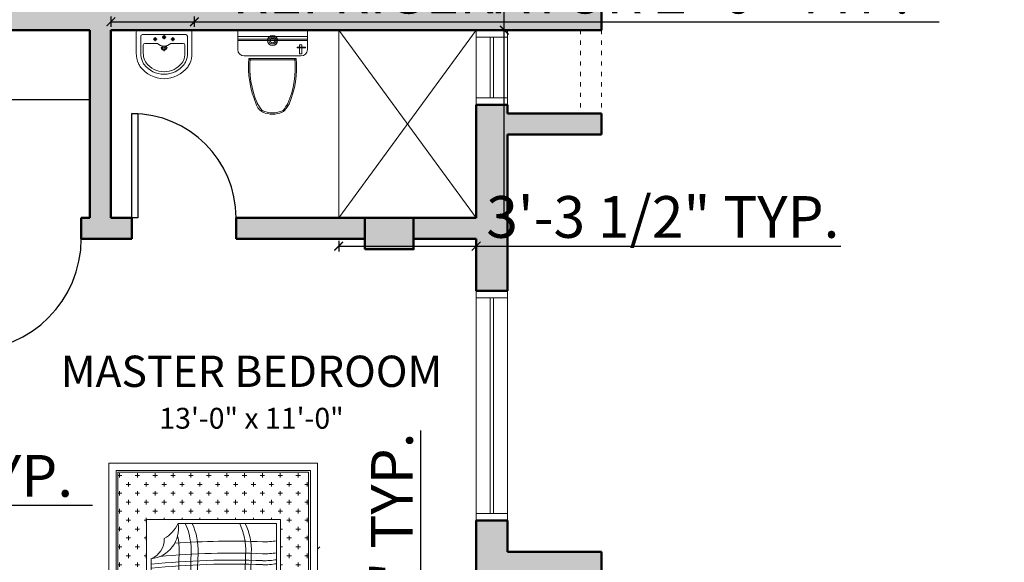
# Model space of a CAD drawing. Units: inches. Extents: x 375 to 1122, y 27 to 1069.
# Tile 151 of 155: x 819 to 1102, y 716 to 872. Entities that reach past the tile are written whole.
import ezdxf

# ---------------------------------------------------------------- set-up
doc = ezdxf.new("R2010")
doc.units = ezdxf.units.IN
doc.linetypes.add('ACAD_ISO03W100', pattern=[30, 12, -18])
for name, color, linetype, lineweight in [('A-ANNO-DIMS', 2, 'Continuous', 18), ('A-AREA-IDEN', 7, 'Continuous', 18), ('A-COLS-PATT', 10, 'Continuous', 13), ('A-FLOR-FIXT', 55, 'Continuous', 18), ('A-FLOR-MILL', 55, 'Continuous', 25), ('A-WALL-OVHD', 77, 'ACAD_ISO03W100', 18), ('A-WALL-PATT', 252, 'Continuous', 13), ('Columns', 10, 'Continuous', 50), ('Doors', 150, 'Continuous', 25), ('Furniture', 30, 'Continuous', 18), ('Shower Areas', 53, 'Continuous', 18), ('Walls', 250, 'Continuous', 50), ('Windows', 122, 'Continuous', 18)]:
    doc.layers.add(name, color=color, linetype=linetype, lineweight=lineweight)
doc.styles.get("Standard").update_dxf_attribs({"font": 'arial.ttf'})
doc.dimstyles.new('ISO-25', dxfattribs={"dimtxt": 12, "dimasz": 2.5, "dimexe": 1.5, "dimexo": 1.5, "dimtad": 1, "dimdec": 1, "dimlunit": 3, "dimtxsty": 'Standard', "dimblk": 'ARCHTICK', "dimcen": 2.5, "dimadec": 0, "dimazin": 0, "dimtfac": 1, "dimtdec": 1, "dimtmove": 0, "dimatfit": 3, "dimfxl": 1.5, "dimfxlon": 1, "dimarcsym": 0})

# ---------------------------------------------------------------- blocks, each defined once
blk = doc.blocks.new('*U2')
for p, q in [((0, 0), (0, 4)), ((32, 0), (32, 4))]:
    blk.add_line(p, q)
blk.add_lwpolyline([(0, 0), (0, -32), (1.75, -32), (1.75, 0)], close=True)
blk.add_arc((0, 0), 32, 270, 0)
blk = doc.blocks.new('*U3')
for p, q in [((0, 0), (0, -4)), ((30, 0), (30, -4))]:
    blk.add_line(p, q)
blk.add_lwpolyline([(0, 0), (0, 30), (1.75, 30), (1.75, 0)], close=True)
blk.add_arc((0, 0), 30, 0, 90)
blk = doc.blocks.new('A$C52B64FF5')
for p, q in [((0.522, 2.628), (0, 2.628)), ((0, 2.628), (0, 2.178)), ((0.262, 2.403), (0.262, 2.616)), ((0.522, 2.178), (0.522, 2.628)), ((2.022, 2.628), (0.522, 2.628)), ((0.522, 2.628), (0.522, 0.628)), ((2.543, 2.628), (2.022, 2.628)), ((2.022, 0.628), (2.022, 2.628)), ((2.022, 2.628), (2.022, 2.178)), ((2.282, 2.403), (2.282, 2.616)), ((2.543, 2.178), (2.543, 2.628)), ((0.721, 2.493), (0.692, 2.493)), ((0.692, 2.493), (0.692, 2.353)), ((0.721, 2.353), (0.721, 2.493)), ((1.767, 2.353), (1.767, 2.493)), ((1.767, 2.493), (1.796, 2.493)), ((1.796, 2.493), (1.796, 2.353)), ((0.263, 2.403), (0.023, 2.403)), ((0.023, 2.403), (0.5, 2.403)), ((0.263, 2.195), (0.263, 2.403)), ((0.692, 2.353), (0.721, 2.353)), ((1.796, 2.353), (1.767, 2.353)), ((2.52, 2.403), (2.043, 2.403)), ((2.28, 2.213), (2.28, 2.403)), ((2.28, 2.403), (2.52, 2.403)), ((0.575, 1.068), (0.575, 2.254)), ((0.575, 2.254), (1.978, 2.254)), ((1.978, 2.254), (1.978, 0.675)), ((0, 2.178), (0.522, 2.178)), ((0.093, 2.178), (0.101, 2.17)), ((0.101, 0), (0.101, 2.178)), ((0.181, 0.08), (0.181, 2.178)), ((0.201, 0.1), (0.201, 2.178)), ((0.201, 2.136), (0.245, 2.136)), ((0.22, 2.111), (0.22, 2.161)), ((0.395, 2.136), (0.445, 2.136)), ((0.42, 2.111), (0.42, 2.161)), ((2.543, 2.178), (2.022, 2.178)), ((2.022, 2.178), (2.543, 2.178)), ((2.022, 2.136), (2.045, 2.136)), ((2.195, 2.136), (2.245, 2.136)), ((2.22, 2.111), (2.22, 2.161)), ((2.337, 2.178), (2.337, 0.1)), ((2.357, 2.178), (2.357, 0.08)), ((2.437, 2.178), (2.437, 0)), ((0.295, 2.036), (0.345, 2.036)), ((0.32, 2.011), (0.32, 2.061)), ((0.495, 2.036), (0.522, 2.036)), ((0.52, 2.011), (0.52, 2.061)), ((2.095, 2.036), (2.145, 2.036)), ((2.12, 2.011), (2.12, 2.061)), ((2.295, 2.036), (2.337, 2.036)), ((2.32, 2.011), (2.32, 2.061)), ((0.201, 1.936), (0.245, 1.936)), ((0.22, 1.911), (0.22, 1.961)), ((0.395, 1.936), (0.445, 1.936)), ((0.42, 1.911), (0.42, 1.961)), ((2.022, 1.936), (2.045, 1.936)), ((2.195, 1.936), (2.245, 1.936)), ((2.22, 1.911), (2.22, 1.961)), ((0.295, 1.836), (0.345, 1.836)), ((0.32, 1.811), (0.32, 1.861)), ((0.495, 1.836), (0.522, 1.836)), ((0.52, 1.811), (0.52, 1.861)), ((2.095, 1.836), (2.145, 1.836)), ((2.12, 1.811), (2.12, 1.861)), ((2.295, 1.836), (2.337, 1.836)), ((2.32, 1.811), (2.32, 1.861)), ((0.201, 1.736), (0.245, 1.736)), ((0.22, 1.711), (0.22, 1.761)), ((0.32, 1.611), (0.32, 1.661)), ((0.395, 1.736), (0.445, 1.736)), ((0.42, 1.711), (0.42, 1.761)), ((0.52, 1.611), (0.52, 1.661)), ((2.022, 1.736), (2.045, 1.736)), ((2.12, 1.611), (2.12, 1.661)), ((2.195, 1.736), (2.245, 1.736)), ((2.22, 1.711), (2.22, 1.761)), ((2.32, 1.611), (2.32, 1.661)), ((0.22, 1.511), (0.22, 1.561)), ((0.295, 1.636), (0.345, 1.636)), ((0.42, 1.511), (0.42, 1.561)), ((0.495, 1.636), (0.522, 1.636)), ((2.095, 1.636), (2.145, 1.636)), ((2.22, 1.511), (2.22, 1.561)), ((2.295, 1.636), (2.337, 1.636)), ((0.201, 1.536), (0.245, 1.536)), ((0.295, 1.436), (0.345, 1.436)), ((0.32, 1.411), (0.32, 1.461)), ((0.395, 1.536), (0.445, 1.536)), ((0.495, 1.436), (0.522, 1.436)), ((0.52, 1.411), (0.52, 1.461)), ((2.022, 1.536), (2.045, 1.536)), ((2.095, 1.436), (2.145, 1.436)), ((2.12, 1.411), (2.12, 1.461)), ((2.195, 1.536), (2.245, 1.536)), ((2.295, 1.436), (2.337, 1.436)), ((2.32, 1.411), (2.32, 1.461)), ((0.201, 1.336), (0.245, 1.336)), ((0.22, 1.311), (0.22, 1.361)), ((0.395, 1.336), (0.445, 1.336)), ((0.42, 1.311), (0.42, 1.361)), ((2.022, 1.336), (2.045, 1.336)), ((2.195, 1.336), (2.245, 1.336)), ((2.22, 1.311), (2.22, 1.361)), ((0.295, 1.236), (0.345, 1.236)), ((0.32, 1.211), (0.32, 1.261)), ((0.495, 1.236), (0.522, 1.236)), ((0.52, 1.211), (0.52, 1.261)), ((2.095, 1.236), (2.145, 1.236)), ((2.12, 1.211), (2.12, 1.261)), ((2.295, 1.236), (2.337, 1.236)), ((2.32, 1.211), (2.32, 1.261)), ((0.201, 1.136), (0.245, 1.136)), ((0.22, 1.111), (0.22, 1.161)), ((0.395, 1.136), (0.445, 1.136)), ((0.42, 1.111), (0.42, 1.161)), ((2.022, 1.136), (2.045, 1.136)), ((2.195, 1.136), (2.245, 1.136)), ((2.22, 1.111), (2.22, 1.161)), ((0.295, 1.036), (0.345, 1.036)), ((0.32, 1.011), (0.32, 1.061)), ((0.495, 1.036), (0.522, 1.036)), ((0.52, 1.011), (0.52, 1.061)), ((2.095, 1.036), (2.145, 1.036)), ((2.12, 1.011), (2.12, 1.061)), ((2.295, 1.036), (2.337, 1.036)), ((2.32, 1.011), (2.32, 1.061)), ((0.201, 0.936), (0.245, 0.936)), ((0.22, 0.911), (0.22, 0.961)), ((0.395, 0.936), (0.445, 0.936)), ((0.42, 0.911), (0.42, 0.961)), ((2.022, 0.936), (2.045, 0.936)), ((2.195, 0.936), (2.245, 0.936)), ((2.22, 0.911), (2.22, 0.961)), ((2.437, 0.962), (2.464, 0.935)), ((0.295, 0.836), (0.345, 0.836)), ((0.32, 0.811), (0.32, 0.861)), ((0.495, 0.836), (0.522, 0.836)), ((0.52, 0.811), (0.52, 0.861)), ((2.095, 0.836), (2.145, 0.836)), ((2.12, 0.811), (2.12, 0.861)), ((2.295, 0.836), (2.337, 0.836)), ((2.32, 0.811), (2.32, 0.861)), ((0.201, 0.736), (0.245, 0.736)), ((0.22, 0.711), (0.22, 0.761)), ((0.395, 0.736), (0.445, 0.736)), ((0.42, 0.711), (0.42, 0.761)), ((1.978, 0.675), (0.876, 0.675)), ((2.022, 0.736), (2.045, 0.736)), ((2.195, 0.736), (2.245, 0.736)), ((2.22, 0.711), (2.22, 0.761)), ((0.22, 0.511), (0.22, 0.561)), ((0.295, 0.636), (0.345, 0.636)), ((0.32, 0.611), (0.32, 0.661)), ((0.42, 0.511), (0.42, 0.561)), ((0.495, 0.636), (0.522, 0.636)), ((0.52, 0.611), (0.52, 0.661)), ((0.522, 0.628), (2.022, 0.628)), ((0.62, 0.511), (0.62, 0.561)), ((0.72, 0.611), (0.72, 0.628)), ((0.82, 0.511), (0.82, 0.561)), ((0.92, 0.611), (0.92, 0.628)), ((1.02, 0.511), (1.02, 0.561)), ((1.12, 0.611), (1.12, 0.628)), ((1.22, 0.511), (1.22, 0.561)), ((1.32, 0.611), (1.32, 0.628)), ((1.42, 0.511), (1.42, 0.561)), ((1.52, 0.611), (1.52, 0.628)), ((1.62, 0.511), (1.62, 0.561)), ((1.72, 0.611), (1.72, 0.628)), ((1.82, 0.511), (1.82, 0.561)), ((1.92, 0.611), (1.92, 0.628)), ((2.02, 0.511), (2.02, 0.561)), ((2.095, 0.636), (2.145, 0.636)), ((2.12, 0.611), (2.12, 0.661)), ((2.22, 0.511), (2.22, 0.561)), ((2.295, 0.636), (2.337, 0.636)), ((2.32, 0.611), (2.32, 0.661)), ((0.201, 0.536), (0.245, 0.536)), ((0.32, 0.411), (0.32, 0.461)), ((0.395, 0.536), (0.445, 0.536)), ((0.52, 0.411), (0.52, 0.461)), ((0.595, 0.536), (0.645, 0.536)), ((0.72, 0.411), (0.72, 0.461)), ((0.795, 0.536), (0.845, 0.536)), ((0.92, 0.411), (0.92, 0.461)), ((0.995, 0.536), (1.045, 0.536)), ((1.12, 0.411), (1.12, 0.461)), ((1.195, 0.536), (1.245, 0.536)), ((1.32, 0.411), (1.32, 0.461)), ((1.395, 0.536), (1.445, 0.536)), ((1.52, 0.411), (1.52, 0.461)), ((1.595, 0.536), (1.645, 0.536)), ((1.72, 0.411), (1.72, 0.461)), ((1.795, 0.536), (1.845, 0.536)), ((1.92, 0.411), (1.92, 0.461)), ((1.995, 0.536), (2.045, 0.536)), ((2.12, 0.411), (2.12, 0.461)), ((2.195, 0.536), (2.245, 0.536)), ((2.32, 0.411), (2.32, 0.461)), ((0.201, 0.336), (0.245, 0.336)), ((0.22, 0.311), (0.22, 0.361)), ((0.295, 0.436), (0.345, 0.436)), ((0.395, 0.336), (0.445, 0.336)), ((0.42, 0.311), (0.42, 0.361)), ((0.495, 0.436), (0.545, 0.436)), ((0.595, 0.336), (0.645, 0.336)), ((0.62, 0.311), (0.62, 0.361)), ((0.695, 0.436), (0.745, 0.436)), ((0.795, 0.336), (0.845, 0.336)), ((0.82, 0.311), (0.82, 0.361)), ((0.895, 0.436), (0.945, 0.436)), ((0.995, 0.336), (1.045, 0.336)), ((1.02, 0.311), (1.02, 0.361)), ((1.095, 0.436), (1.145, 0.436)), ((1.195, 0.336), (1.245, 0.336)), ((1.22, 0.311), (1.22, 0.361)), ((1.295, 0.436), (1.345, 0.436)), ((1.395, 0.336), (1.445, 0.336)), ((1.42, 0.311), (1.42, 0.361)), ((1.495, 0.436), (1.545, 0.436)), ((1.595, 0.336), (1.645, 0.336)), ((1.62, 0.311), (1.62, 0.361)), ((1.695, 0.436), (1.745, 0.436)), ((1.795, 0.336), (1.845, 0.336)), ((1.82, 0.311), (1.82, 0.361)), ((1.895, 0.436), (1.945, 0.436)), ((1.995, 0.336), (2.045, 0.336)), ((2.02, 0.311), (2.02, 0.361)), ((2.095, 0.436), (2.145, 0.436)), ((2.195, 0.336), (2.245, 0.336)), ((2.22, 0.311), (2.22, 0.361)), ((2.295, 0.436), (2.337, 0.436)), ((0.295, 0.236), (0.345, 0.236)), ((0.32, 0.211), (0.32, 0.261)), ((0.495, 0.236), (0.545, 0.236)), ((0.52, 0.211), (0.52, 0.261)), ((0.695, 0.236), (0.745, 0.236)), ((0.72, 0.211), (0.72, 0.261)), ((0.895, 0.236), (0.945, 0.236)), ((0.92, 0.211), (0.92, 0.261)), ((1.095, 0.236), (1.145, 0.236)), ((1.12, 0.211), (1.12, 0.261)), ((1.295, 0.236), (1.345, 0.236)), ((1.32, 0.211), (1.32, 0.261)), ((1.495, 0.236), (1.545, 0.236)), ((1.52, 0.211), (1.52, 0.261)), ((1.695, 0.236), (1.745, 0.236)), ((1.72, 0.211), (1.72, 0.261)), ((1.895, 0.236), (1.945, 0.236)), ((1.92, 0.211), (1.92, 0.261)), ((2.095, 0.236), (2.145, 0.236)), ((2.12, 0.211), (2.12, 0.261)), ((2.295, 0.236), (2.337, 0.236)), ((2.32, 0.211), (2.32, 0.261)), ((0.201, 0.136), (0.245, 0.136)), ((0.22, 0.111), (0.22, 0.161)), ((0.395, 0.136), (0.445, 0.136)), ((0.42, 0.111), (0.42, 0.161)), ((0.595, 0.136), (0.645, 0.136)), ((0.62, 0.111), (0.62, 0.161)), ((0.795, 0.136), (0.845, 0.136)), ((0.82, 0.111), (0.82, 0.161)), ((0.995, 0.136), (1.045, 0.136)), ((1.02, 0.111), (1.02, 0.161)), ((1.195, 0.136), (1.245, 0.136)), ((1.22, 0.111), (1.22, 0.161)), ((1.395, 0.136), (1.445, 0.136)), ((1.42, 0.111), (1.42, 0.161)), ((1.595, 0.136), (1.645, 0.136)), ((1.62, 0.111), (1.62, 0.161)), ((1.795, 0.136), (1.845, 0.136)), ((1.82, 0.111), (1.82, 0.161)), ((1.995, 0.136), (2.045, 0.136)), ((2.02, 0.111), (2.02, 0.161)), ((2.195, 0.136), (2.245, 0.136)), ((2.22, 0.111), (2.22, 0.161)), ((2.437, 0), (0.101, 0)), ((2.357, 0.08), (0.181, 0.08)), ((2.337, 0.1), (0.201, 0.1))]:
    blk.add_line(p, q)
for centre, radius in [((0.263, 2.403), 0.163), ((0.263, 2.403), 0.143), ((2.28, 2.403), 0.163), ((2.28, 2.403), 0.143)]:
    blk.add_circle(centre, radius)
for centre, radius, start, end in [((0.752, 2.492), 0.101, 192.774, 239.2386), ((0.757, 2.452), 0.0808, 161.4559, 221.5545), ((1.736, 2.492), 0.101, 300.7614, 347.226), ((1.732, 2.452), 0.0808, 318.4455, 18.5441), ((0.689, 2.306), 0.098, 80.9486, 149.4879), ((0.644, 2.315), 0.107, 59.2174, 107.2401), ((0.665, 2.321), 0.0913, 67.8398, 120.4859), ((0.729, 2.33), 0.0776, 109.2642, 192.2669), ((1.759, 2.33), 0.0776, 347.7331, 73.8836), ((1.799, 2.306), 0.098, 30.5121, 99.0514), ((1.844, 2.315), 0.107, 72.7599, 120.7826), ((1.823, 2.321), 0.0913, 59.5141, 112.1602), ((9.729, 1.341), 8.848, 174.0754, 182.1662), ((9.863, 1.341), 8.848, 174.0754, 182.1662), ((9.941, 1.341), 8.848, 174.0754, 182.1662), ((10.474, 1.341), 8.848, 174.0754, 182.1662), ((10.537, 1.341), 8.848, 174.0754, 182.1662), ((1.488, 10.589), 8.848, 264.0754, 272.1662), ((1.488, 10.57), 8.848, 264.0754, 272.1662), ((1.488, 10.526), 8.848, 264.0754, 272.1662), ((1.85, 1.028), 0.72, 79.7409, 92.1662), ((1.85, 1.01), 0.72, 79.7409, 92.1662), ((1.85, 0.965), 0.72, 79.7409, 92.1662), ((1.488, 10.447), 8.848, 264.0754, 272.1662), ((1.85, 0.887), 0.72, 79.7409, 92.1662), ((1.488, 10.313), 8.848, 264.0754, 272.1662), ((1.85, 0.753), 0.72, 79.7409, 92.1662), ((1.488, 9.976), 8.848, 264.0754, 272.1662), ((1.488, 9.932), 8.848, 264.0754, 272.1662), ((1.85, 0.416), 0.72, 79.7409, 92.1662), ((0.487, 0.852), 0.234, 358.0368, 67.7864), ((0.539, 0.729), 0.342, 350.9267, 83.9565), ((1.488, 9.854), 8.848, 264.7058, 272.1662), ((0.169, 0.979), 0.72, 346.8653, 2.1662), ((0.303, 0.979), 0.72, 334.9836, 2.1662), ((0.381, 0.979), 0.72, 334.9836, 2.1662), ((0.913, 0.979), 0.72, 334.9836, 2.1662), ((0.976, 0.979), 0.72, 334.9836, 2.1662), ((1.85, 0.371), 0.72, 79.7409, 92.1662), ((1.85, 0.293), 0.72, 79.7409, 92.1662), ((1.488, 9.72), 8.848, 265.7785, 272.1662), ((0.528, 0.51), 0.385, 25.3912, 60.0686), ((1.85, 0.159), 0.72, 79.7409, 92.1662)]:
    blk.add_arc(centre, radius, start, end)
for points, knots in [([(0.737, 2.429), (0.734, 2.439), (0.724, 2.472), (0.715, 2.518), (0.741, 2.546), (0.909, 2.551), (1.086, 2.559), (1.264, 2.536), (1.298, 2.532)], [0, 0, 0, 0, 0.0298664, 0.1071619, 0.1152509, 0.1416099, 0.5761797, 0.6768951, 0.6768951, 0.6768951, 0.6768951]), ([(1.195, 2.544), (1.285, 2.549), (1.448, 2.559), (1.628, 2.543), (1.718, 2.544), (1.735, 2.544)], [0, 0, 0, 0, 0.2717358, 0.4891854, 0.5406465, 0.5406465, 0.5406465, 0.5406465]), ([(1.735, 2.544), (1.742, 2.532), (1.759, 2.501), (1.758, 2.462), (1.735, 2.382), (1.745, 2.415), (1.749, 2.426)], [0, 0, 0, 0, 0.0383771, 0.1013156, 0.1484959, 0.1756343, 0.1756343, 0.1756343, 0.1756343]), ([(1.08, 2.318), (1.023, 2.316), (0.91, 2.312), (0.791, 2.299), (0.723, 2.328), (0.731, 2.377), (0.735, 2.409), (0.737, 2.429)], [0, 0, 0, 0, 0.1744349, 0.3406483, 0.347042, 0.3874998, 0.4538558, 0.4538558, 0.4538558, 0.4538558]), ([(1.749, 2.426), (1.753, 2.408), (1.76, 2.375), (1.757, 2.336), (1.744, 2.306), (1.668, 2.315), (1.559, 2.311), (1.403, 2.312), (1.305, 2.33), (1.263, 2.338)], [0, 0, 0, 0, 0.0550284, 0.1011576, 0.1178362, 0.1437253, 0.3009935, 0.4726259, 0.6000038, 0.6000038, 0.6000038, 0.6000038]), ([(1.375, 2.318), (1.295, 2.315), (1.168, 2.311), (1.041, 2.32), (0.995, 2.323)], [0, 0, 0, 0, 0.2401688, 0.38052, 0.38052, 0.38052, 0.38052])]:
    blk.add_open_spline(points, degree=3, knots=knots)
blk = doc.blocks.new('A$C00C51FE0')
at = {"ltscale": 2}
for p, q in [((16.79, 8.49), (3.21, 8.49)), ((1.59, 4.18), (1.59, 6.81)), ((1.59, 6.81), (2.25, 6.81)), ((1.85, 7.41), (18.15, 7.41)), ((2.25, 6.81), (2.25, 4.18)), ((16.79, 8.12), (3.21, 8.12)), ((0, 0), (0, 5.56)), ((20, 2.96), (0, 2.96)), ((0.5, 4.84), (0.5, 5.06)), ((0.5, 5.06), (2.91, 5.06)), ((2.91, 4.84), (0.5, 4.84)), ((2.25, 4.18), (1.59, 4.18)), ((2.91, 5.06), (2.91, 4.84)), ((20, 5.56), (20, 0)), ((20, 2.59), (0, 2.59)), ((20, 1.85), (0, 1.85)), ((20, 0), (0, 0))]:
    blk.add_line(p, q, dxfattribs=at)
for radius in [1.44, 1.07, 0.698]:
    blk.add_circle((10, 2.96), radius, dxfattribs=at)
for centre, radius, start, end in [((22.68, 10.69), 20.34, 142.816, 148.8373), ((22.68, 10.69), 19.97, 141.7352, 148.8373), ((7.96, 21.86), 1.85, 112.9199, 142.816), ((10, 17.03), 6.73, 63.5839, 116.4161), ((10, 17.03), 7.1, 67.0801, 112.9199), ((11.04, 20.15), 3.83, 16.1902, 63.2078), ((-2.68, 10.69), 19.97, 31.1627, 38.2648), ((29.69, 10.65), 26.6, 156.5869, 185.4494), ((29.69, 10.65), 26.23, 156.5869, 185.4494), ((-9.69, 10.65), 26.23, 354.5506, 23.4131), ((-9.69, 10.65), 26.6, 354.5506, 23.4131), ((1.85, 5.56), 1.85, 90, 180), ((18.15, 5.56), 1.85, 0, 90)]:
    blk.add_arc(centre, radius, start, end, dxfattribs=at)
blk = doc.blocks.new('WINDOW-21_5IN')
for p, q in [((4, 2), (4, 19.5)), ((5, 2), (5, 19.5))]:
    blk.add_line(p, q)
blk.add_lwpolyline([(0, 0), (9, 0), (9, 21.5), (0, 21.5)], close=True)
for points in [[(9, 19.5), (0, 19.5)], [(0, 2), (9, 2)]]:
    blk.add_lwpolyline(points)
blk = doc.blocks.new('LAVATORY-16IN')
for p, q in [((1.27, 7.37), (1.27, 12.19)), ((1.78, 12.7), (14.22, 12.7)), ((4.89, 11.37), (6.03, 11.37)), ((5.46, 10.79), (5.46, 11.94)), ((7.43, 11.94), (8.57, 11.94)), ((8, 11.37), (8, 12.51)), ((9.97, 11.37), (11.11, 11.37)), ((10.54, 10.79), (10.54, 11.94)), ((14.73, 12.19), (14.73, 7.37)), ((2.01, 7.37), (2.01, 9.65)), ((2.51, 10.16), (6.08, 10.16)), ((7.02, 8.89), (8.98, 8.89)), ((8, 7.91), (8, 9.4)), ((9.91, 10.16), (13.49, 10.16)), ((13.99, 9.65), (13.99, 7.37))]:
    blk.add_line(p, q)
blk.add_lwpolyline([(0.51, 13.97), (15.49, 13.97, -0.414214), (16, 13.46), (16, 7.37, -0.104704), (15.37, 4.36, -0.038376), (14.78, 3.36, -0.495903), (1.22, 3.36, -0.038376), (0.63, 4.36, -0.104704), (0, 7.37), (0, 13.46, -0.414214)], format="xyb", close=True)
for points in [[(1.27, 7.37, 0.102694), (1.78, 4.92, 0.037256), (2.25, 4.11, 0.085618)], [(2.01, 7.37, 0.101044), (2.44, 5.24, 0.036381), (2.84, 4.54, 0.084644)], [(13.16, 4.54, 0.036381), (13.56, 5.24, 0.101044), (13.99, 7.37, 0.11083)], [(13.75, 4.11, 0.037256), (14.22, 4.92, 0.102694), (14.73, 7.37, 0.111333)]]:
    blk.add_lwpolyline(points, format="xyb")
for centre, radius in [((5.46, 11.37), 0.381), ((8, 11.94), 0.444), ((10.54, 11.37), 0.381), ((8, 8.89), 0.508)]:
    blk.add_circle(centre, radius)
for centre, radius, start, end in [((1.78, 12.19), 0.508, 90, 180), ((14.22, 12.19), 0.508, 0, 90), ((2.51, 9.65), 0.508, 90, 180), ((7.99, 12.19), 2.79, 226.6581, 313.3419), ((8, 8.89), 0.762, 133.135, 47.0367), ((13.49, 9.65), 0.508, 0, 90), ((8, 8.52), 7.25, 217.471, 322.529), ((8, 8.52), 6.51, 217.6433, 322.3567)]:
    blk.add_arc(centre, radius, start, end)
blk = doc.blocks.new('COLUMN-14X9IN')
blk.add_lwpolyline([(0, 0), (14, 0), (14, 9), (0, 9)], close=True)
blk = doc.blocks.new('SHOWER-PAN-39_5X54IN')
for p, q in [((0, 0), (39.5, 54)), ((0, 54), (39.5, 0.05))]:
    blk.add_line(p, q)
blk.add_lwpolyline([(39.5, 54), (0, 54), (0, 0), (39.5, 0)], close=True)
blk = doc.blocks.new('_ArchTick')
at = {"color": 0, "linetype": 'ByBlock', "const_width": 0.15}
blk.add_lwpolyline([(-0.5, -0.5), (0.5, 0.5)], dxfattribs=at)
blk = doc.blocks.new('*D42')
at = {"layer": 'A-ANNO-DIMS', "color": 0, "lineweight": -2, "transparency": 16777216}
for p, q in [((934.11, 676.53), (934.11, 753.42)), ((933.51, 676.53), (935.61, 676.53)), ((934.11, 667.53), (934.11, 676.53)), ((933.51, 667.53), (935.61, 667.53))]:
    blk.add_line(p, q, dxfattribs=at)
at = {"layer": 'Defpoints', "color": 0, "transparency": 16777216}
for p in [(932.01, 676.53), (934.11, 676.53), (932.01, 667.53)]:
    blk.add_point(p, dxfattribs=at)
at = {"layer": 'A-ANNO-DIMS', "color": 0, "lineweight": -2, "transparency": 16777216, "xscale": 2.5, "yscale": 2.5, "zscale": 2.5}
for p, rotation in [((934.11, 676.53), 90), ((934.11, 667.53), 270)]:
    blk.add_blockref('_ArchTick', p, dxfattribs=dict(at, rotation=rotation))
at = {"layer": 'A-ANNO-DIMS', "color": 0, "transparency": 16777216, "insert": (927.36, 716.23), "char_height": 12, "attachment_point": 5, "rotation": 90}
blk.add_mtext('0\'-9" TYP.', dxfattribs=at)
blk = doc.blocks.new('*D57')
at = {"layer": 'A-ANNO-DIMS', "color": 0, "lineweight": -2, "transparency": 16777216}
for p, q in [((512.46, 733.49), (512.46, 730.49)), ((638.07, 733.49), (638.07, 730.49)), ((512.46, 731.99), (638.07, 731.99)), ((638.07, 731.99), (839.76, 731.99))]:
    blk.add_line(p, q, dxfattribs=at)
at = {"layer": 'Defpoints', "color": 0, "transparency": 16777216}
for p in [(512.46, 750.84), (638.07, 750.84), (638.07, 731.99)]:
    blk.add_point(p, dxfattribs=at)
at = {"layer": 'A-ANNO-DIMS', "color": 0, "lineweight": -2, "transparency": 16777216, "xscale": 2.5, "yscale": 2.5, "zscale": 2.5, "rotation": 180}
blk.add_blockref('_ArchTick', (512.46, 731.99), dxfattribs=at)
at = {"layer": 'A-ANNO-DIMS', "color": 0, "lineweight": -2, "transparency": 16777216, "xscale": 2.5, "yscale": 2.5, "zscale": 2.5}
blk.add_blockref('_ArchTick', (638.07, 731.99), dxfattribs=at)
at = {"layer": 'A-ANNO-DIMS', "color": 0, "transparency": 16777216, "insert": (740.16, 738.83), "char_height": 12, "attachment_point": 5}
blk.add_mtext('SOFA SET 10\'-5 1/2" TYP.', dxfattribs=at)
blk = doc.blocks.new('*D61')
at = {"layer": 'A-ANNO-DIMS', "color": 0, "lineweight": -2, "transparency": 16777216}
for p, q in [((845.01, 872.43), (845.01, 869.43)), ((869.01, 872.43), (869.01, 869.43)), ((845.01, 870.93), (869.01, 870.93)), ((869.01, 870.93), (1083.13, 870.93))]:
    blk.add_line(p, q, dxfattribs=at)
at = {"layer": 'Defpoints', "color": 0, "transparency": 16777216}
for p in [(845.01, 874.53), (869.01, 874.53), (869.01, 870.93)]:
    blk.add_point(p, dxfattribs=at)
at = {"layer": 'A-ANNO-DIMS', "color": 0, "lineweight": -2, "transparency": 16777216, "xscale": 2.5, "yscale": 2.5, "zscale": 2.5, "rotation": 180}
blk.add_blockref('_ArchTick', (845.01, 870.93), dxfattribs=at)
at = {"layer": 'A-ANNO-DIMS', "color": 0, "lineweight": -2, "transparency": 16777216, "xscale": 2.5, "yscale": 2.5, "zscale": 2.5}
blk.add_blockref('_ArchTick', (869.01, 870.93), dxfattribs=at)
at = {"layer": 'A-ANNO-DIMS', "color": 0, "transparency": 16777216, "insert": (977.32, 877.76), "char_height": 12, "attachment_point": 5}
blk.add_mtext('REFRIGERATOR 2\'-0" TYP.', dxfattribs=at)
blk = doc.blocks.new('*D75')
at = {"layer": 'A-ANNO-DIMS', "color": 0, "lineweight": -2, "transparency": 16777216}
for p, q in [((958.11, 868.53), (958.11, 1064.59)), ((956.61, 868.53), (959.61, 868.53)), ((958.11, 814.53), (958.11, 868.53)), ((956.61, 814.53), (959.61, 814.53))]:
    blk.add_line(p, q, dxfattribs=at)
at = {"layer": 'Defpoints', "color": 0, "transparency": 16777216}
for p in [(950.01, 868.53), (958.11, 868.53), (950.01, 814.53)]:
    blk.add_point(p, dxfattribs=at)
at = {"layer": 'A-ANNO-DIMS', "color": 0, "lineweight": -2, "transparency": 16777216, "xscale": 2.5, "yscale": 2.5, "zscale": 2.5}
for p, rotation in [((958.11, 868.53), 90), ((958.11, 814.53), 270)]:
    blk.add_blockref('_ArchTick', p, dxfattribs=dict(at, rotation=rotation))
at = {"layer": 'A-ANNO-DIMS', "color": 0, "transparency": 16777216, "insert": (951.27, 967.81), "char_height": 12, "attachment_point": 5, "rotation": 90}
blk.add_mtext('SHOWER PAN 4\'-6" TYP.', dxfattribs=at)
blk = doc.blocks.new('*D76')
at = {"layer": 'A-ANNO-DIMS', "color": 0, "lineweight": -2, "transparency": 16777216}
for p, q in [((910.51, 807.93), (910.51, 804.93)), ((950.01, 807.93), (950.01, 804.93)), ((910.51, 806.43), (950.01, 806.43)), ((950.01, 806.43), (1054.86, 806.43))]:
    blk.add_line(p, q, dxfattribs=at)
at = {"layer": 'Defpoints', "color": 0, "transparency": 16777216}
for p in [(910.51, 814.53), (950.01, 814.53), (950.01, 806.43)]:
    blk.add_point(p, dxfattribs=at)
at = {"layer": 'A-ANNO-DIMS', "color": 0, "lineweight": -2, "transparency": 16777216, "xscale": 2.5, "yscale": 2.5, "zscale": 2.5, "rotation": 180}
blk.add_blockref('_ArchTick', (910.51, 806.43), dxfattribs=at)
at = {"layer": 'A-ANNO-DIMS', "color": 0, "lineweight": -2, "transparency": 16777216, "xscale": 2.5, "yscale": 2.5, "zscale": 2.5}
blk.add_blockref('_ArchTick', (950.01, 806.43), dxfattribs=at)
at = {"layer": 'A-ANNO-DIMS', "color": 0, "transparency": 16777216, "insert": (1003.68, 813.26), "char_height": 12, "attachment_point": 5}
blk.add_mtext('3\'-3 1/2" TYP.', dxfattribs=at)
blk = doc.blocks.new('*D77')
at = {"layer": 'A-ANNO-DIMS', "color": 0, "lineweight": -2, "transparency": 16777216}
for p, q in [((812.01, 892.38), (812.01, 889.38)), ((923.01, 892.38), (923.01, 889.38)), ((812.01, 890.88), (923.01, 890.88)), ((923.01, 890.88), (1101.82, 890.88))]:
    blk.add_line(p, q, dxfattribs=at)
at = {"layer": 'Defpoints', "color": 0, "transparency": 16777216}
for p in [(812.01, 907.53), (923.01, 907.53), (923.01, 890.88)]:
    blk.add_point(p, dxfattribs=at)
at = {"layer": 'A-ANNO-DIMS', "color": 0, "lineweight": -2, "transparency": 16777216, "xscale": 2.5, "yscale": 2.5, "zscale": 2.5, "rotation": 180}
blk.add_blockref('_ArchTick', (812.01, 890.88), dxfattribs=at)
at = {"layer": 'A-ANNO-DIMS', "color": 0, "lineweight": -2, "transparency": 16777216, "xscale": 2.5, "yscale": 2.5, "zscale": 2.5}
blk.add_blockref('_ArchTick', (923.01, 890.88), dxfattribs=at)
at = {"layer": 'A-ANNO-DIMS', "color": 0, "transparency": 16777216, "insert": (1013.66, 897.72), "char_height": 12, "attachment_point": 5}
blk.add_mtext('L-COUNTER 9\'-3" TYP.', dxfattribs=at)
blk = doc.blocks.new('*D84')
at = {"layer": 'A-ANNO-DIMS', "color": 0, "lineweight": -2, "transparency": 16777216}
for p, q in [((845.01, 117.53), (845.01, 114.53)), ((950.01, 117.53), (950.01, 114.53)), ((845.01, 116.03), (950.01, 116.03))]:
    blk.add_line(p, q, dxfattribs=at)
at = {"layer": 'Defpoints', "color": 0, "transparency": 16777216}
for p in [(845.01, 814.53), (950.01, 814.53), (950.01, 116.03)]:
    blk.add_point(p, dxfattribs=at)
at = {"layer": 'A-ANNO-DIMS', "color": 0, "lineweight": -2, "transparency": 16777216, "xscale": 2.5, "yscale": 2.5, "zscale": 2.5, "rotation": 180}
blk.add_blockref('_ArchTick', (845.01, 116.03), dxfattribs=at)
at = {"layer": 'A-ANNO-DIMS', "color": 0, "lineweight": -2, "transparency": 16777216, "xscale": 2.5, "yscale": 2.5, "zscale": 2.5}
blk.add_blockref('_ArchTick', (950.01, 116.03), dxfattribs=at)
at = {"layer": 'A-ANNO-DIMS', "color": 0, "transparency": 16777216, "insert": (897.51, 122.78), "char_height": 12, "attachment_point": 5}
blk.add_mtext('8\'-9"', dxfattribs=at)
blk = doc.blocks.new('*D85')
at = {"layer": 'A-ANNO-DIMS', "color": 0, "lineweight": -2, "transparency": 16777216}
for p, q in [((401.51, 868.53), (398.51, 868.53)), ((400.01, 814.53), (400.01, 868.53)), ((401.51, 814.53), (398.51, 814.53))]:
    blk.add_line(p, q, dxfattribs=at)
at = {"layer": 'Defpoints', "color": 0, "transparency": 16777216}
for p in [(400.01, 868.53), (845.01, 868.53), (845.01, 814.53)]:
    blk.add_point(p, dxfattribs=at)
at = {"layer": 'A-ANNO-DIMS', "color": 0, "lineweight": -2, "transparency": 16777216, "xscale": 2.5, "yscale": 2.5, "zscale": 2.5}
for p, rotation in [((400.01, 868.53), 90), ((400.01, 814.53), 270)]:
    blk.add_blockref('_ArchTick', p, dxfattribs=dict(at, rotation=rotation))
at = {"layer": 'A-ANNO-DIMS', "color": 0, "transparency": 16777216, "insert": (393.26, 841.53), "char_height": 12, "attachment_point": 5, "rotation": 90}
blk.add_mtext('4\'-6"', dxfattribs=at)
blk = doc.blocks.new('*D88')
at = {"layer": 'A-ANNO-DIMS', "color": 0, "lineweight": -2, "transparency": 16777216}
for p, q in [((731.01, 1052.53), (731.01, 1055.53)), ((731.01, 1054.03), (854.01, 1054.03)), ((854.01, 1052.53), (854.01, 1055.53))]:
    blk.add_line(p, q, dxfattribs=at)
at = {"layer": 'Defpoints', "color": 0, "transparency": 16777216}
for p in [(854.01, 1054.03), (731.01, 502.53), (854.01, 502.53)]:
    blk.add_point(p, dxfattribs=at)
at = {"layer": 'A-ANNO-DIMS', "color": 0, "lineweight": -2, "transparency": 16777216, "xscale": 2.5, "yscale": 2.5, "zscale": 2.5, "rotation": 180}
blk.add_blockref('_ArchTick', (731.01, 1054.03), dxfattribs=at)
at = {"layer": 'A-ANNO-DIMS', "color": 0, "lineweight": -2, "transparency": 16777216, "xscale": 2.5, "yscale": 2.5, "zscale": 2.5}
blk.add_blockref('_ArchTick', (854.01, 1054.03), dxfattribs=at)
at = {"layer": 'A-ANNO-DIMS', "color": 0, "transparency": 16777216, "insert": (792.51, 1060.78), "char_height": 12, "attachment_point": 5}
blk.add_mtext('10\'-3"', dxfattribs=at)

msp = doc.modelspace()

# ---------------------------------------------------------------- hatches: boundary and pattern name
at = {"layer": 'A-COLS-PATT'}
h = msp.add_hatch(color=256, dxfattribs=at)
h.dxf.hatch_style = 1
h.paths.add_polyline_path([(512.51, 982.53), (498.51, 982.53), (498.51, 973.53), (512.51, 973.53)])
h.paths.add_polyline_path([(666.51, 982.53), (652.51, 982.53), (652.51, 973.53), (666.51, 973.53)])
h.paths.add_polyline_path([(802.01, 982.53), (788.01, 982.53), (788.01, 973.53), (802.01, 973.53)])
h.paths.add_polyline_path([(932.01, 982.53), (918.01, 982.53), (918.01, 973.53), (932.01, 973.53)])
h.paths.add_polyline_path([(507.51, 841.53), (498.51, 841.53), (498.51, 827.53), (507.51, 827.53)])
h.paths.add_polyline_path([(666.51, 844.53), (652.51, 844.53), (652.51, 835.53), (666.51, 835.53)])
h.paths.add_polyline_path([(802.01, 814.53), (788.01, 814.53), (788.01, 805.53), (802.01, 805.53)])
h.paths.add_polyline_path([(932.01, 814.53), (918.01, 814.53), (918.01, 805.53), (932.01, 805.53)])
h.paths.add_polyline_path([(507.51, 719.53), (498.51, 719.53), (498.51, 705.53), (507.51, 705.53)])
h.paths.add_polyline_path([(731.01, 676.53), (722.01, 676.53), (722.01, 662.53), (731.01, 662.53)])
h.paths.add_polyline_path([(802.01, 676.53), (788.01, 676.53), (788.01, 667.53), (802.01, 667.53)])
h.paths.add_polyline_path([(932.01, 676.53), (918.01, 676.53), (918.01, 667.53), (932.01, 667.53)])
h.paths.add_polyline_path([(932.01, 583.53), (918.01, 583.53), (918.01, 574.53), (932.01, 574.53)])
h.paths.add_polyline_path([(868.01, 583.53), (854.01, 583.53), (854.01, 574.53), (868.01, 574.53)])
h.paths.add_polyline_path([(868.01, 502.53), (854.01, 502.53), (854.01, 493.53), (868.01, 493.53)])
h.paths.add_polyline_path([(932.01, 502.53), (918.01, 502.53), (918.01, 493.53), (932.01, 493.53)])
h.paths.add_polyline_path([(672.51, 592.03), (663.51, 592.03), (663.51, 578.03), (672.51, 578.03)])
h.paths.add_polyline_path([(512.51, 589.53), (498.51, 589.53), (498.51, 580.53), (512.51, 580.53)])
h.paths.add_polyline_path([(507.51, 464.53), (498.51, 464.53), (498.51, 450.53), (507.51, 450.53)])
h.paths.add_polyline_path([(731.01, 507.53), (722.01, 507.53), (722.01, 493.53), (731.01, 493.53)])
h.paths.add_polyline_path([(802.01, 502.53), (788.01, 502.53), (788.01, 493.53), (802.01, 493.53)])
h.paths.add_polyline_path([(507.51, 342.53), (498.51, 342.53), (498.51, 328.53), (507.51, 328.53)])
h.paths.add_polyline_path([(512.51, 196.53), (498.51, 196.53), (498.51, 187.53), (512.51, 187.53)])
h.paths.add_polyline_path([(666.51, 334.53), (652.51, 334.53), (652.51, 325.53), (666.51, 325.53)])
h.paths.add_polyline_path([(666.51, 196.53), (652.51, 196.53), (652.51, 187.53), (666.51, 187.53)])
h.paths.add_polyline_path([(805.01, 196.53), (791.01, 196.53), (791.01, 187.53), (805.01, 187.53)])
h.paths.add_polyline_path([(932.01, 196.53), (918.01, 196.53), (918.01, 187.53), (932.01, 187.53)])
h.paths.add_polyline_path([(932.01, 334.53), (918.01, 334.53), (918.01, 325.53), (932.01, 325.53)])
h.paths.add_polyline_path([(805.01, 334.53), (791.01, 334.53), (791.01, 325.53), (805.01, 325.53)])
at = {"layer": 'A-WALL-PATT'}
h = msp.add_hatch(color=256, dxfattribs=at)
h.dxf.hatch_style = 1
h.paths.add_polyline_path([(962.01, 388.53), (989.01, 388.53), (989.01, 394.53), (962.01, 394.53), (932.01, 394.53), (932.01, 397.53), (923.01, 397.53), (923.01, 394.53), (842.01, 394.53), (842.01, 334.53), (839.51, 334.53), (839.51, 328.53), (854.01, 328.53), (854.01, 334.53), (848.01, 334.53), (848.01, 388.53), (953.01, 388.53), (953.01, 356.08), (962.01, 356.08), (962.01, 358.55), (989.01, 358.55), (989.01, 364.55), (962.01, 364.55)])
h.paths.add_polyline_path([(989.01, 502.53), (932.01, 502.53), (932.01, 583.53), (932.01, 593.53), (923.01, 593.53), (923.01, 583.53), (854.01, 583.53), (854.01, 556.53), (863.01, 556.53), (863.01, 574.53), (923.01, 574.53), (923.01, 502.53), (863.01, 502.53), (863.01, 520.53), (854.01, 520.53), (854.01, 502.53), (773.01, 502.53), (773.01, 493.53), (788.01, 493.53), (788.01, 402.03), (722.01, 402.03), (722.01, 373.53), (728.01, 373.53), (728.01, 396.03), (788.01, 396.03), (788.01, 373.53), (794.01, 373.53), (794.01, 430.53), (814.01, 430.53), (814.01, 436.53), (794.01, 436.53), (794.01, 493.53), (923.01, 493.53), (923.01, 487.53), (932.01, 487.53), (932.01, 493.53), (983.01, 493.53), (983.01, 473.53), (989.01, 473.53)])
h.paths.add_polyline_path([(797.01, 325.53), (805.01, 325.53), (805.01, 328.53), (807.51, 328.53), (807.51, 334.53), (791.01, 334.53), (791.01, 226.53), (770.76, 226.53), (770.76, 217.53), (791.01, 217.53), (791.01, 187.53), (855.01, 187.53), (855.01, 196.53), (797.01, 196.53)])
h.paths.add_polyline_path([(989.01, 238.53), (962.01, 238.53), (962.01, 256.42), (953.01, 256.42), (953.01, 229.53), (980.01, 229.53), (980.01, 196.53), (915.01, 196.53), (915.01, 187.53), (989.01, 187.53)])
h.paths.add_polyline_path([(962.01, 334.53), (884.01, 334.53), (884.01, 328.53), (918.01, 328.53), (918.01, 325.53), (932.01, 325.53), (932.01, 328.53), (953.01, 328.53), (953.01, 304.42), (962.01, 304.42)])
h.paths.add_polyline_path([(606.51, 283.53), (609.51, 283.53), (609.51, 289.53), (600.51, 289.53), (600.51, 196.53), (578.51, 196.53), (578.51, 187.53), (606.51, 187.53), (606.51, 196.53)])
h.paths.add_polyline_path([(666.51, 292.53), (660.51, 292.53), (660.51, 289.53), (633.51, 289.53), (633.51, 283.53), (660.51, 283.53), (660.51, 196.53), (628.01, 196.53), (628.01, 187.53), (630.53, 187.53), (630.53, 160.53), (636.53, 160.53), (636.53, 187.53), (660.51, 187.53), (660.51, 160.53), (666.51, 160.53), (666.51, 217.53), (686.76, 217.53), (686.76, 226.53), (666.51, 226.53)])
h.paths.add_polyline_path([(480.51, 256.42), (471.51, 256.42), (471.51, 238.53), (444.51, 238.53), (444.51, 187.53), (518.51, 187.53), (518.51, 196.53), (453.51, 196.53), (453.51, 229.53), (480.51, 229.53)])
h.paths.add_polyline_path([(480.51, 328.53), (652.51, 328.53), (652.51, 325.53), (660.51, 325.53), (660.51, 322.53), (666.51, 322.53), (666.51, 334.53), (507.51, 334.53), (507.51, 360.53), (498.51, 360.53), (498.51, 334.53), (471.51, 334.53), (471.51, 304.42), (480.51, 304.42)])
h.paths.add_polyline_path([(507.51, 484.53), (498.51, 484.53), (498.51, 444.53), (507.51, 444.53), (507.51, 454.53), (621.51, 454.53), (621.51, 460.53), (507.51, 460.53)])
h.paths.add_polyline_path([(672.51, 604.53), (683.26, 604.53), (683.26, 613.53), (669.51, 613.53), (669.51, 649.53), (663.51, 649.53), (663.51, 589.53), (507.51, 589.53), (507.51, 613.53), (498.51, 613.53), (498.51, 556.53), (507.51, 556.53), (507.51, 580.53), (663.51, 580.53), (663.51, 520.53), (669.51, 520.53), (669.51, 556.53), (683.26, 556.53), (683.26, 565.53), (672.51, 565.53)])
h.paths.add_polyline_path([(731.01, 667.53), (734.01, 667.53), (734.01, 676.53), (728.01, 676.53), (728.01, 715.53), (657.51, 715.53), (657.51, 709.53), (663.51, 709.53), (663.51, 673.53), (669.51, 673.53), (669.51, 709.53), (722.01, 709.53), (722.01, 613.53), (704.76, 613.53), (704.76, 604.53), (722.01, 604.53), (722.01, 565.53), (704.76, 565.53), (704.76, 556.53), (722.01, 556.53), (722.01, 502.53), (722.01, 460.53), (669.51, 460.53), (669.51, 496.53), (663.51, 496.53), (663.51, 460.53), (657.51, 460.53), (657.51, 454.53), (728.01, 454.53), (728.01, 493.53), (734.01, 493.53), (734.01, 502.53), (731.01, 502.53)])
h.paths.add_polyline_path([(986.01, 718.53), (959.01, 718.53), (959.01, 727.53), (950.01, 727.53), (950.01, 709.53), (977.01, 709.53), (977.01, 676.53), (794.01, 676.53), (794.01, 805.53), (802.01, 805.53), (802.01, 808.53), (804.51, 808.53), (804.51, 814.53), (788.01, 814.53), (788.01, 774.03), (728.01, 774.03), (728.01, 796.53), (722.01, 796.53), (722.01, 768.03), (788.01, 768.03), (788.01, 676.53), (773.01, 676.53), (773.01, 667.53), (923.01, 667.53), (923.01, 657.53), (932.01, 657.53), (932.01, 667.53), (986.01, 667.53)])
h.paths.add_polyline_path([(621.51, 715.53), (507.51, 715.53), (507.51, 733.53), (498.51, 733.53), (498.51, 715.53), (498.51, 685.53), (507.51, 685.53), (507.51, 709.53), (621.51, 709.53)])
h.paths.add_polyline_path([(666.51, 847.03), (660.51, 847.03), (660.51, 844.53), (652.51, 844.53), (652.51, 841.53), (480.51, 841.53), (480.51, 859.53), (471.51, 859.53), (471.51, 835.53), (498.51, 835.53), (498.51, 817.53), (507.51, 817.53), (507.51, 835.53), (666.51, 835.53)])
h.paths.add_polyline_path([(480.51, 940.53), (453.51, 940.53), (453.51, 973.53), (518.51, 973.53), (518.51, 982.53), (444.51, 982.53), (444.51, 931.53), (471.51, 931.53), (471.51, 907.53), (480.51, 907.53)])
h.paths.add_polyline_path([(606.51, 982.53), (578.51, 982.53), (578.51, 973.53), (600.51, 973.53), (600.51, 880.53), (609.51, 880.53), (609.51, 886.53), (606.51, 886.53)])
h.paths.add_polyline_path([(666.51, 943.53), (686.76, 943.53), (686.76, 952.53), (666.51, 952.53), (666.51, 1009.53), (660.51, 1009.53), (660.51, 982.53), (636.53, 982.53), (636.53, 1009.53), (630.53, 1009.53), (630.53, 982.53), (628.01, 982.53), (628.01, 973.53), (660.51, 973.53), (660.51, 886.53), (633.51, 886.53), (633.51, 880.53), (660.51, 880.53), (660.51, 877.03), (666.51, 877.03)])
h.paths.add_polyline_path([(986.01, 874.53), (932.01, 874.53), (932.01, 877.53), (923.01, 877.53), (923.01, 874.53), (788.01, 874.53), (788.01, 868.53), (788.01, 844.53), (794.01, 844.53), (794.01, 868.53), (839.01, 868.53), (839.01, 814.53), (836.51, 814.53), (836.51, 808.53), (851.01, 808.53), (851.01, 814.53), (845.01, 814.53), (845.01, 868.53), (986.01, 868.53)])
h.paths.add_polyline_path([(959.01, 838.55), (986.01, 838.55), (986.01, 844.55), (959.01, 844.55), (959.01, 847.03), (950.01, 847.03), (950.01, 814.53), (881.01, 814.53), (881.01, 808.53), (918.01, 808.53), (918.01, 805.53), (932.01, 805.53), (932.01, 808.53), (950.01, 808.53), (950.01, 793.53), (959.01, 793.53)])
h.paths.add_polyline_path([(986.01, 982.53), (899.01, 982.53), (899.01, 973.53), (923.01, 973.53), (923.01, 967.53), (932.01, 967.53), (932.01, 973.53), (980.01, 973.53), (980.01, 953.53), (986.01, 953.53)])
h.paths.add_polyline_path([(851.01, 982.53), (788.01, 982.53), (788.01, 952.53), (770.76, 952.53), (770.76, 943.53), (788.01, 943.53), (788.01, 910.53), (814.01, 910.53), (814.01, 916.53), (794.01, 916.53), (794.01, 973.53), (851.01, 973.53)])

# ---------------------------------------------------------------- linework, layer by layer
at = {"layer": 'A-FLOR-MILL'}
msp.add_line((839.01, 848.53), (794.01, 848.53), dxfattribs=at)
at = {"layer": 'A-WALL-OVHD', "ltscale": 0.1}
for p, q in [((980.01, 868.53), (980.01, 844.55)), ((986.01, 868.53), (986.01, 844.55))]:
    msp.add_line(p, q, dxfattribs=at)
at = {"layer": 'Walls'}
for p, q in [((986.01, 874.53), (986.01, 868.53)), ((839.01, 868.53), (794.01, 868.53)), ((839.01, 868.53), (839.01, 814.53)), ((845.01, 868.53), (845.01, 814.53)), ((986.01, 868.53), (845.01, 868.53)), ((950.01, 847.03), (950.01, 814.53)), ((959.01, 847.03), (950.01, 847.03)), ((959.01, 847.03), (959.01, 844.55)), ((986.01, 844.55), (959.01, 844.55)), ((986.01, 838.55), (986.01, 844.55)), ((959.01, 838.55), (959.01, 793.53)), ((959.01, 838.55), (986.01, 838.55)), ((836.51, 814.53), (836.51, 808.53)), ((839.01, 814.53), (836.51, 814.53)), ((851.01, 814.53), (845.01, 814.53)), ((851.01, 814.53), (851.01, 808.53)), ((950.01, 814.53), (881.01, 814.53)), ((881.01, 814.53), (881.01, 808.53)), ((851.01, 808.53), (836.51, 808.53)), ((918.01, 808.53), (881.01, 808.53)), ((918.01, 808.53), (918.01, 805.53)), ((950.01, 808.53), (932.01, 808.53)), ((932.01, 805.53), (932.01, 808.53)), ((950.01, 808.53), (950.01, 793.53)), ((918.01, 805.53), (932.01, 805.53)), ((959.01, 793.53), (950.01, 793.53)), ((959.01, 727.53), (950.01, 727.53)), ((950.01, 727.53), (950.01, 709.53)), ((959.01, 727.53), (959.01, 718.53)), ((986.01, 718.53), (959.01, 718.53)), ((986.01, 667.53), (986.01, 718.53))]:
    msp.add_line(p, q, dxfattribs=at)
at = {"layer": 'Windows'}
for p, q in [((954.01, 729.53), (954.01, 791.53)), ((955.01, 729.53), (955.01, 791.53))]:
    msp.add_line(p, q, dxfattribs=at)
msp.add_lwpolyline([(950.01, 793.53), (959.01, 793.53), (959.01, 727.53), (950.01, 727.53)], close=True, dxfattribs=at)
for points in [[(950.01, 791.53), (959.01, 791.53)], [(959.01, 729.53), (950.01, 729.53)]]:
    msp.add_lwpolyline(points, dxfattribs=at)

# ---------------------------------------------------------------- block references
at = {"layer": 'A-FLOR-FIXT'}
msp.add_blockref('LAVATORY-16IN', (852.32, 854.56), dxfattribs=at)
at = {"layer": 'A-FLOR-FIXT', "rotation": 180}
msp.add_blockref('A$C00C51FE0', (901.51, 868.5), dxfattribs=at)
at = {"layer": 'Columns'}
msp.add_blockref('COLUMN-14X9IN', (918.01, 805.53), dxfattribs=at)
at = {"layer": 'Doors'}
for name, p in [('*U3', (851.01, 814.53)), ('*U2', (804.51, 808.53))]:
    msp.add_blockref(name, p, dxfattribs=at)
at = {"layer": 'Furniture', "xscale": -25.67804170018038, "yscale": 25.67804170018038, "zscale": 25.67804170018038, "rotation": 180}
msp.add_blockref('A$C52B64FF5', (841.85, 744), dxfattribs=at)
at = {"layer": 'Shower Areas'}
msp.add_blockref('SHOWER-PAN-39_5X54IN', (910.51, 814.53), dxfattribs=at)
at = {"layer": 'Windows'}
msp.add_blockref('WINDOW-21_5IN', (950.01, 847.03), dxfattribs=at)

# ---------------------------------------------------------------- texts
at = {"layer": 'A-AREA-IDEN', "insert": (823.51, 753.94), "char_height": 12, "attachment_point": 7}
msp.add_mtext_dynamic_manual_height_columns('\\pxqc;{\\fArial|b1|i0|c0|p34;\\H0.75x;MASTER BEDROOM\\H1.33333x;\\P\\fArial|b0|i0|c0|p34;\\H0.5x;13\'-0" x 11\'-0"}', width=123.8705, gutter_width=12.5, heights=[0], dxfattribs=at)

# ---------------------------------------------------------------- dimensions: what is measured, and where the dimension line sits
at = {"layer": 'A-ANNO-DIMS'}
for base, p1, p2, picture, middle in [((854.01, 1054.03), (731.01, 502.53), (854.01, 502.53), '*D88', (792.51, 1060.78)), ((950.01, 116.03), (845.01, 814.53), (950.01, 814.53), '*D84', (897.51, 122.78))]:
    dim = msp.add_linear_dim(base=base, p1=p1, p2=p2, dimstyle='ISO-25', override={"dimdec": 1, "dimlfac": 1, "dimrnd": 0, "dimzin": 1, "dimdsep": 46, "dimlunit": 4, "dimfrac": 2}, dxfattribs=at)
    dim.commit()
    dim.dimension.update_dxf_attribs({"geometry": picture, "text_midpoint": middle})
for base, p1, p2, text, picture, middle in [((958.11, 868.53), (950.01, 814.53), (950.01, 868.53), 'SHOWER PAN <> TYP.', '*D75', (951.27, 967.81)), ((934.11, 676.53), (932.01, 667.53), (932.01, 676.53), '<> TYP.', '*D42', (927.36, 716.23))]:
    dim = msp.add_linear_dim(base=base, p1=p1, p2=p2, angle=90, text=text, dimstyle='ISO-25', override={"dimdec": 1, "dimlfac": 1, "dimrnd": 0, "dimzin": 1, "dimdsep": 46, "dimlunit": 4, "dimfrac": 2}, dxfattribs=at)
    dim.commit()
    dim.dimension.update_dxf_attribs({"geometry": picture, "text_midpoint": middle})
for base, p1, p2, text, picture, middle in [((923.01, 890.88), (812.01, 907.53), (923.01, 907.53), 'L-COUNTER <> TYP.', '*D77', (1013.66, 897.72)), ((869.01, 870.93), (845.01, 874.53), (869.01, 874.53), 'REFRIGERATOR <> TYP.', '*D61', (977.32, 877.76)), ((950.01, 806.43), (910.51, 814.53), (950.01, 814.53), '<> TYP.', '*D76', (1003.68, 813.26)), ((638.07, 731.99), (512.46, 750.84), (638.07, 750.84), 'SOFA SET <> TYP.', '*D57', (740.16, 738.83))]:
    dim = msp.add_linear_dim(base=base, p1=p1, p2=p2, text=text, dimstyle='ISO-25', override={"dimdec": 1, "dimlfac": 1, "dimrnd": 0, "dimzin": 1, "dimdsep": 46, "dimlunit": 4, "dimfrac": 2}, dxfattribs=at)
    dim.commit()
    dim.dimension.update_dxf_attribs({"geometry": picture, "text_midpoint": middle})
dim = msp.add_linear_dim(base=(400.01, 868.53), p1=(845.01, 814.53), p2=(845.01, 868.53), angle=90, dimstyle='ISO-25', override={"dimdec": 1, "dimlfac": 1, "dimrnd": 0, "dimzin": 1, "dimdsep": 46, "dimlunit": 4, "dimfrac": 2}, dxfattribs=at)
dim.commit()
dim.dimension.update_dxf_attribs({"geometry": '*D85', "text_midpoint": (393.26, 841.53)})

doc.saveas('drawing.dxf')
